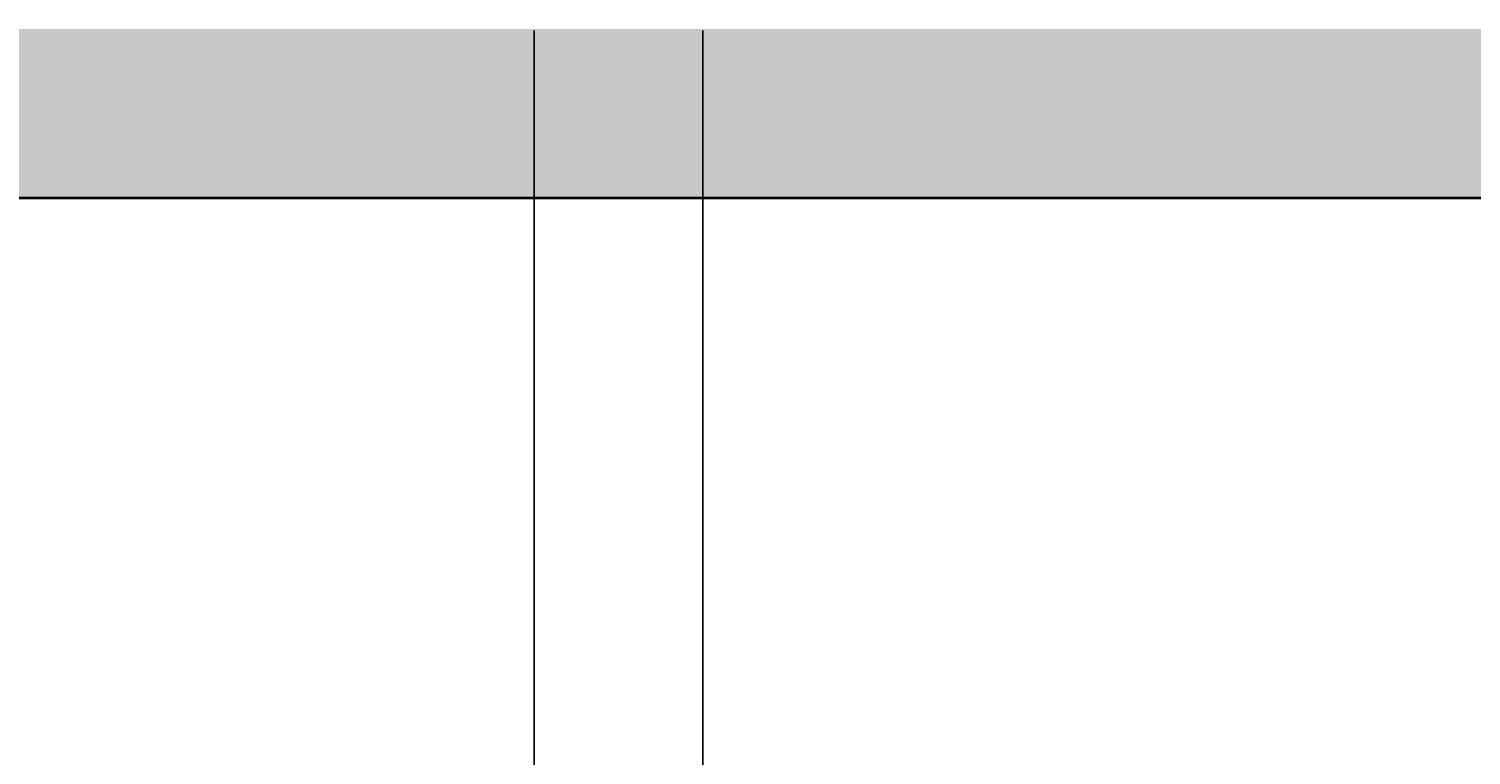
# Model space of a CAD drawing. Units: inches. Extents: x 2549 to 3108, y 1683 to 2362.
# Tile 15 of 30: x 2711 to 2762, y 2055 to 2081. Entities that reach past the tile are written whole.
import ezdxf

# ---------------------------------------------------------------- set-up
doc = ezdxf.new("R2010")
doc.units = ezdxf.units.IN
for name, color, linetype, lineweight in [('A-ANNO-DIMS', 2, 'Continuous', 18), ('A-WALL', 7, 'Continuous', 35), ('A-WALL-PATT', 89, 'Continuous', 13)]:
    doc.layers.add(name, color=color, linetype=linetype, lineweight=lineweight)
doc.layers.add('C-PKNG-VEHI-PATT', color=251, linetype='Continuous', lineweight=13, true_color=0x636466)
doc.layers.add('C-PVMT-PATT', color=9, linetype='Continuous', lineweight=13, true_color=0xc7c8ca)
doc.styles.get("Standard").update_dxf_attribs({"font": 'arial.ttf'})
doc.dimstyles.get("Standard").update_dxf_attribs({"dimtxt": 0.18, "dimasz": 0.18, "dimexe": 0.18, "dimexo": 0.0625, "dimgap": 0.09, "dimtad": 0, "dimtih": 1, "dimtoh": 1, "dimdec": 4, "dimzin": 0, "dimdsep": 46, "dimtxsty": 'Standard', "dimcen": 0.09, "dimadec": 0, "dimazin": 0, "dimtfac": 1, "dimtdec": 4, "dimtofl": 0, "dimtmove": 0, "dimatfit": 3, "dimfxl": 1, "dimtolj": 1, "dimtzin": 0, "dimarcsym": 0})

# ---------------------------------------------------------------- blocks, each defined once
blk = doc.blocks.new('*D42')
at = {"layer": 'A-ANNO-DIMS', "color": 0, "lineweight": -2, "transparency": 16777216}
for p, q in [((2638.643, 2080.461), (2638.643, 1683.444)), ((2728.643, 2080.461), (2728.643, 1683.444)), ((2638.823, 1683.624), (2683.424, 1683.624)), ((2728.463, 1683.624), (2683.861, 1683.624))]:
    blk.add_line(p, q, dxfattribs=at)
at = {"layer": 'A-ANNO-DIMS', "color": 0, "transparency": 16777216}
for points in [[(2638.823, 1683.654), (2638.823, 1683.594), (2638.643, 1683.624)], [(2728.463, 1683.654), (2728.463, 1683.594), (2728.643, 1683.624)]]:
    blk.add_solid(points, dxfattribs=at)
at = {"layer": 'Defpoints', "color": 0, "transparency": 16777216}
for p in [(2638.643, 2080.524), (2728.643, 2080.524), (2728.643, 1683.624)]:
    blk.add_point(p, dxfattribs=at)
at = {"layer": 'A-ANNO-DIMS', "color": 0, "transparency": 16777216, "insert": (2683.643, 1683.624), "char_height": 0.18, "attachment_point": 5}
blk.add_mtext('\\A1;90', dxfattribs=at)
blk = doc.blocks.new('*D43')
at = {"layer": 'A-ANNO-DIMS', "color": 0, "lineweight": -2, "transparency": 16777216}
for p, q in [((2734.643, 2080.461), (2734.643, 1683.444)), ((2806.643, 2080.461), (2806.643, 1683.444)), ((2734.823, 1683.624), (2770.425, 1683.624)), ((2806.463, 1683.624), (2770.86, 1683.624))]:
    blk.add_line(p, q, dxfattribs=at)
at = {"layer": 'A-ANNO-DIMS', "color": 0, "transparency": 16777216}
for points in [[(2734.823, 1683.654), (2734.823, 1683.594), (2734.643, 1683.624)], [(2806.463, 1683.654), (2806.463, 1683.594), (2806.643, 1683.624)]]:
    blk.add_solid(points, dxfattribs=at)
at = {"layer": 'Defpoints', "color": 0, "transparency": 16777216}
for p in [(2734.643, 2080.524), (2806.643, 2080.524), (2806.643, 1683.624)]:
    blk.add_point(p, dxfattribs=at)
at = {"layer": 'A-ANNO-DIMS', "color": 0, "transparency": 16777216, "insert": (2770.643, 1683.624), "char_height": 0.18, "attachment_point": 5}
blk.add_mtext('\\A1;72', dxfattribs=at)
blk = doc.blocks.new('*D59')
at = {"layer": 'A-ANNO-DIMS', "color": 0, "lineweight": -2, "transparency": 16777216}
for p, q in [((2680.978, 1761.586), (2680.978, 2362.323)), ((2786.158, 1761.586), (2786.158, 2362.323)), ((2681.158, 2362.143), (2733.112, 2362.143)), ((2785.978, 2362.143), (2734.023, 2362.143))]:
    blk.add_line(p, q, dxfattribs=at)
at = {"layer": 'A-ANNO-DIMS', "color": 0, "transparency": 16777216}
for points in [[(2681.158, 2362.173), (2681.158, 2362.113), (2680.978, 2362.143)], [(2785.978, 2362.173), (2785.978, 2362.113), (2786.158, 2362.143)]]:
    blk.add_solid(points, dxfattribs=at)
at = {"layer": 'Defpoints', "color": 0, "transparency": 16777216}
for p in [(2786.158, 2362.143), (2680.978, 1761.524), (2786.158, 1761.524)]:
    blk.add_point(p, dxfattribs=at)
at = {"layer": 'A-ANNO-DIMS', "color": 0, "transparency": 16777216, "insert": (2733.568, 2362.143), "char_height": 0.18, "attachment_point": 5}
blk.add_mtext('\\A1;105.18', dxfattribs=at)

msp = doc.modelspace()

# ---------------------------------------------------------------- hatches: boundary and pattern name
at = {"layer": 'A-WALL-PATT'}
h = msp.add_hatch(color=256, dxfattribs=at)
h.dxf.hatch_style = 1
h.paths.add_polyline_path([(2638.6427, 2272.5237), (3034.6427, 2272.5237), (3034.6427, 1936.5237), (3043.6427, 1936.5237), (3043.6427, 2281.5237), (2629.6427, 2281.5237), (2629.6427, 2074.5237), (2812.6427, 2074.5237), (2812.6427, 2140.5237), (2785.7177, 2140.5237), (2785.7177, 2134.5237), (2806.6427, 2134.5237), (2806.6427, 2080.5237), (2638.6427, 2080.5237)])
h.paths.add_polyline_path([(2638.6427, 1972.5237), (2662.6427, 1972.5237), (2662.6427, 2041.0557), (2653.6427, 2041.0557), (2653.6427, 1978.5237), (2629.6427, 1978.5237), (2629.6427, 1795.5237), (2662.6427, 1795.5237), (2881.6427, 1795.5237), (2881.6427, 1936.5237), (2965.9351, 1936.5237), (2965.9351, 1974.5439), (2959.9351, 1974.5439), (2959.9351, 1945.5237), (2881.6427, 1945.5237), (2872.6427, 1945.5237), (2872.6427, 1804.5237), (2662.6427, 1804.5237), (2638.6427, 1804.5237)])
at = {"layer": 'C-PKNG-VEHI-PATT'}
h = msp.add_hatch(color=256, dxfattribs=at)
h.dxf.hatch_style = 1
edge = h.paths.add_edge_path()
edge.add_ellipse((2935.7258, 1791.964), major_axis=(-50.66, 0), ratio=0.8423039, start_angle=248.16505, end_angle=265.72258)
edge.add_line((2938.911, 1834.5507), (2925.8653, 1834.5507))
edge.add_ellipse((2929.0505, 1791.964), major_axis=(50.66, 0), ratio=0.8423039, start_angle=94.27742, end_angle=111.83495)
edge.add_line((2912.8508, 1832.3947), (2914.2044, 1822.2495))
edge.add_ellipse((2930.6538, 1783.1023), major_axis=(-49.3014, 0), ratio=0.8423039, start_angle=-85.12993, end_angle=-67.20809, ccw=False)
edge.add_line((2927.1247, 1824.5225), (2937.6516, 1824.5225))
edge.add_ellipse((2934.1225, 1783.1023), major_axis=(49.3014, 0), ratio=0.8423039, start_angle=67.20809, end_angle=85.12993, ccw=False)
edge.add_line((2950.5719, 1822.2495), (2951.9255, 1832.3947))
edge = h.paths.add_edge_path()
edge.add_ellipse((2903.4793, 1857.3351), major_axis=(-34.7979, 0), ratio=0.8423039, start_angle=180, end_angle=209.43857)
edge.add_ellipse((2961.297, 1857.3351), major_axis=(34.7979, 0), ratio=0.8423039, start_angle=150.56143, end_angle=180)
edge.add_line((2926.4991, 1857.3351), (2926.4991, 1843.7609))
edge.add_ellipse((2924.1251, 1844.3143), major_axis=(-0.2209, 3.9278), ratio=0.6038336, start_angle=89.00201, end_angle=253.65741, ccw=False)
edge.add_line((2921.7512, 1844.2222), (2921.7512, 1853.3975))
edge.add_line((2921.7512, 1853.3975), (2925.269, 1855.8484))
edge.add_ellipse((2925.4782, 1855.4931), major_axis=(0.4584, 0), ratio=0.8423039, start_angle=90, end_angle=134.48021, ccw=False)
edge.add_line((2925.4782, 1855.8792), (2926.4991, 1855.8792))
edge.add_line((2926.4991, 1855.8792), (2926.4991, 1857.3351))
edge.add_ellipse((2961.297, 1857.3351), major_axis=(34.7979, 0), ratio=0.8423039, start_angle=150.56143, end_angle=180, ccw=False)
edge.add_line((2932.3882, 1873.6501), (2932.3882, 1875.7801))
edge.add_ellipse((2932.3882, 1875.3939), major_axis=(0.4584, 0), ratio=0.8423039, start_angle=90, end_angle=127.93313)
edge.add_line((2932.1366, 1875.7167), (2928.5915, 1873.7564))
edge.add_ellipse((2899.9271, 2002.4692), major_axis=(155.4756, 0), ratio=0.84230387, start_angle=-80.743434, end_angle=-77.445067, ccw=False)
edge.add_ellipse((2949.4402, 1715.2151), major_axis=(-189.1422, 0), ratio=0.84230387, start_angle=-79.790461, end_angle=-77.555373)
edge.add_ellipse((3300.3614, 1852.5642), major_axis=(-386.1662, 0), ratio=0.84230387, start_angle=-2.863715, end_angle=2.198541)
edge.add_ellipse((2929.0505, 1792.5159), major_axis=(-55.6192, 0), ratio=0.8423039, start_angle=-85.91759, end_angle=-72.28005, ccw=False)
edge.add_line((2925.7129, 1839.2798), (2939.0634, 1839.2798))
edge.add_ellipse((2935.7258, 1792.5159), major_axis=(55.6192, 0), ratio=0.8423039, start_angle=72.28005, end_angle=85.91759, ccw=False)
edge.add_ellipse((2564.4149, 1852.5642), major_axis=(-386.1662, 0), ratio=0.84230387, start_angle=177.801459, end_angle=182.863715)
edge.add_ellipse((2915.3361, 1715.2151), major_axis=(189.1422, 0), ratio=0.84230387, start_angle=77.555373, end_angle=79.790461)
edge.add_ellipse((2964.8492, 2002.4692), major_axis=(-155.4756, 0), ratio=0.84230387, start_angle=77.445067, end_angle=80.743434, ccw=False)
edge.add_line((2936.1848, 1873.7564), (2932.6397, 1875.7167))
edge.add_ellipse((2932.3882, 1875.3939), major_axis=(0.4584, 0), ratio=0.8423039, start_angle=52.06687, end_angle=90)
edge.add_line((2932.3882, 1875.7801), (2932.3882, 1873.6501))
edge.add_ellipse((2903.4793, 1857.3351), major_axis=(-34.7979, 0), ratio=0.8423039, start_angle=180, end_angle=209.43857, ccw=False)
edge.add_line((2938.2772, 1857.3351), (2938.2772, 1855.8792))
edge.add_line((2938.2772, 1855.8792), (2939.4059, 1855.8792))
edge.add_ellipse((2939.2981, 1855.4931), major_axis=(-0.4584, 0), ratio=0.8423039, start_angle=225.51979, end_angle=270, ccw=False)
edge.add_line((2939.5903, 1855.7906), (2943.0251, 1853.3975))
edge.add_line((2943.0251, 1853.3975), (2943.0251, 1844.2222))
edge.add_ellipse((2940.6512, 1844.3143), major_axis=(0.2209, 3.9278), ratio=0.6038336, start_angle=106.34259, end_angle=270.99799, ccw=False)
edge.add_line((2938.2772, 1843.7609), (2938.2772, 1857.3351))
edge = h.paths.add_edge_path()
edge.add_ellipse((2932.3882, 1865.1973), major_axis=(91.081, 0), ratio=0.8423039, start_angle=256.401865, end_angle=283.598135, ccw=False)
edge.add_line((2914.2044, 1790.0239), (2914.2044, 1778.3622))
edge.add_ellipse((2932.3882, 1853.5356), major_axis=(91.081, 0), ratio=0.8423039, start_angle=256.401865, end_angle=283.598135)
edge.add_line((2950.5719, 1778.3622), (2950.5719, 1790.0239))
edge = h.paths.add_edge_path()
edge.add_ellipse((2948.7383, 1772.3145), major_axis=(1.8336, 0), ratio=0.8423039, start_angle=0, end_angle=90)
edge.add_line((2948.7383, 1773.859), (2916.038, 1773.859))
edge.add_ellipse((2916.038, 1772.3145), major_axis=(1.8336, 0), ratio=0.8423039, start_angle=90, end_angle=180)
edge.add_line((2914.2044, 1772.3145), (2914.2044, 1760.2558))
edge.add_line((2914.2044, 1760.2558), (2950.5719, 1760.2558))
edge.add_line((2950.5719, 1760.2558), (2950.5719, 1772.3145))
h.paths.add_polyline_path([(2748.8496, 2101.6383), (2798.148, 2101.6383), (2798.148, 2111.4248), (2748.8496, 2111.4248)], flags=9)
h.paths.add_polyline_path([(2685.2081, 2101.489), (2719.3253, 2101.489), (2719.3253, 2111.2819), (2685.2081, 2111.2819)], flags=9)
h.paths.add_polyline_path([(2814.6852, 1907.1328), (2847.8384, 1907.1328), (2847.8384, 1916.9258), (2814.6852, 1916.9258)], flags=9)
h.paths.add_polyline_path([(2814.3906, 1835.5864), (2848.0172, 1835.5864), (2848.0172, 1845.3794), (2814.3906, 1845.3794)], flags=9)
h.paths.add_polyline_path([(2800.5245, 1759.1674), (2853.7435, 1759.1674), (2853.7435, 1768.954), (2800.5245, 1768.954)], flags=9)
h.paths.add_polyline_path([(2972.4611, 1807.3305), (3015.3943, 1807.3305), (3015.3943, 1817.117), (2972.4611, 1817.117)], flags=9)
h.paths.add_polyline_path([(2902.3327, 1888.6731), (2937.9131, 1888.6731), (2937.9131, 1898.4661), (2902.3327, 1898.4661)], flags=9)
h.paths.add_polyline_path([(2712.1779, 1878.9039), (2754.1257, 1878.9039), (2754.1257, 1888.6904), (2712.1779, 1888.6904)], flags=9)
h.paths.add_polyline_path([(2614.0056, 2012.812), (2650.0251, 2012.812), (2650.0251, 2022.4371), (2614.0056, 2022.4371)], flags=9)
h.paths.add_polyline_path([(2713.3129, 2003.1645), (2747.4237, 2003.1645), (2747.4237, 2012.951), (2713.3129, 2012.951)], flags=9)
h.paths.add_polyline_path([(2950.1379, 2001.6934), (2982.2992, 2001.6934), (2982.2992, 2011.48), (2950.1379, 2011.48)], flags=9)
h.paths.add_polyline_path([(2940.864, 2238.5537), (2997.5066, 2238.5537), (2997.5066, 2248.3466), (2940.864, 2248.3466)], flags=9)
h.paths.add_polyline_path([(2821.5457, 2202.8348), (2855.663, 2202.8348), (2855.663, 2212.6278), (2821.5457, 2212.6278)], flags=9)
h.paths.add_polyline_path([(2661.8026, 2238.6249), (2718.4451, 2238.6249), (2718.4451, 2248.4179), (2661.8026, 2248.4179)], flags=9)
at = {"layer": 'C-PVMT-PATT'}
h = msp.add_hatch(color=256, dxfattribs=at)
h.dxf.hatch_style = 1
h.paths.add_polyline_path([(3067.6427, 2305.5237), (2605.6427, 2305.5237), (2605.6427, 2074.5237), (2629.6427, 2074.5237), (2629.6427, 2281.5237), (3043.6427, 2281.5237), (3043.6427, 1885.5237), (3043.6427, 1872.8745), (3031.1672, 1872.8745), (3031.1672, 1862.5731), (2995.8054, 1862.5731), (2995.8054, 1872.8745), (2983.1752, 1872.8745), (2983.1752, 1885.5237), (2881.6427, 1885.5237), (2881.6427, 1795.5237), (2751.0977, 1795.5237), (2751.0977, 1761.5237), (2786.1577, 1761.5237), (2786.1577, 1723.5237), (2881.84, 1723.5237), (2881.84, 1714.5237), (3067.6427, 1714.5237), (3067.6427, 1723.5237)])
edge = h.paths.add_edge_path(flags=16)
edge.add_ellipse((2949.4402, 1710.9683), major_axis=(-194.1014, 0), ratio=0.84230387, start_angle=-77.874034, end_angle=-76.219471, ccw=False)
edge.add_ellipse((2949.4402, 1715.2151), major_axis=(-189.1422, 0), ratio=0.84230387, start_angle=-79.790461, end_angle=-77.555373, ccw=False)
edge.add_ellipse((2899.9271, 2002.4692), major_axis=(155.4756, 0), ratio=0.84230387, start_angle=-80.743434, end_angle=-77.445067)
edge.add_line((2928.5915, 1873.7564), (2932.3882, 1875.8558))
edge.add_line((2932.3882, 1875.8558), (2936.1848, 1873.7564))
edge.add_ellipse((2964.8492, 2002.4692), major_axis=(-155.4756, 0), ratio=0.84230387, start_angle=77.445067, end_angle=80.743434)
edge.add_ellipse((2915.3361, 1715.2151), major_axis=(189.1422, 0), ratio=0.84230387, start_angle=77.555373, end_angle=79.790461, ccw=False)
edge.add_ellipse((2915.3361, 1710.9683), major_axis=(-194.1014, 0), ratio=0.84230387, start_angle=256.219471, end_angle=257.874034, ccw=False)
edge.add_ellipse((2628.2871, 1850.2612), major_axis=(-327.2532, 0), ratio=0.84230387, start_angle=182.17995, end_angle=183.650428, ccw=False)
edge.add_ellipse((2955.5637, 1861.9334), major_axis=(-0.9168, 0), ratio=0.8423039, start_angle=180, end_angle=270, ccw=False)
edge.add_line((2956.4805, 1862.3857), (2956.4805, 1846.4866))
edge.add_ellipse((2955.5637, 1846.939), major_axis=(-0.9168, 0), ratio=0.8423039, start_angle=90, end_angle=180, ccw=False)
edge.add_ellipse((-3607.0606, 1835.832), major_axis=(-6562.6242, 0), ratio=0.84230387, start_angle=179.61613322, end_angle=180.09022909, ccw=False)
edge.add_ellipse((2955.5637, 1791.0926), major_axis=(0.9168, 0), ratio=0.8423039, start_angle=0, end_angle=90, ccw=False)
edge.add_line((2956.4805, 1791.545), (2956.4805, 1775.6459))
edge.add_ellipse((2955.5637, 1776.0982), major_axis=(0.9168, 0), ratio=0.8423039, start_angle=270, end_angle=360, ccw=False)
edge.add_ellipse((-3607.0606, 1835.832), major_axis=(-6562.6242, 0), ratio=0.84230387, start_angle=179.3813568, end_angle=179.47172853, ccw=False)
edge.add_ellipse((2954.5907, 1763.8768), major_axis=(-1.3752, 0), ratio=0.8423039, start_angle=179.37176, end_angle=248.46476, ccw=False)
edge.add_ellipse((-3607.519, 1835.832), major_axis=(-6564.0409, 0), ratio=0.842303863, start_angle=179.35344594, end_angle=179.37176282, ccw=False)
edge.add_ellipse((2952.6829, 1761.8002), major_axis=(3.2503, 0), ratio=0.8423039, start_angle=-90, end_angle=-0.64655, ccw=False)
edge.add_line((2952.6829, 1759.0625), (2912.0934, 1759.0625))
edge.add_ellipse((2912.0934, 1761.8002), major_axis=(3.2503, 0), ratio=0.8423039, start_angle=180.64655, end_angle=270, ccw=False)
edge.add_ellipse((9472.2953, 1835.832), major_axis=(-6564.0409, 0), ratio=0.842303871, start_angle=0.62823722, end_angle=0.6465541, ccw=False)
edge.add_ellipse((2910.1856, 1763.8768), major_axis=(1.3752, 0), ratio=0.8423039, start_angle=111.53524, end_angle=180.62824, ccw=False)
edge.add_ellipse((9471.8369, 1835.832), major_axis=(-6562.6242, 0), ratio=0.84230387, start_angle=0.52827147, end_angle=0.6465541, ccw=False)
edge.add_ellipse((2909.2126, 1776.0982), major_axis=(-0.9168, 0), ratio=0.8423039, start_angle=0, end_angle=90, ccw=False)
edge.add_line((2908.2958, 1775.6459), (2908.2958, 1791.545))
edge.add_ellipse((2909.2126, 1791.0926), major_axis=(-0.9168, 0), ratio=0.8423039, start_angle=-90, end_angle=0, ccw=False)
edge.add_ellipse((9471.8369, 1835.832), major_axis=(-6562.6242, 0), ratio=0.84230387, start_angle=-0.09022909, end_angle=0.38386678, ccw=False)
edge.add_ellipse((2909.2126, 1846.939), major_axis=(-0.9168, 0), ratio=0.8423039, start_angle=0, end_angle=90, ccw=False)
edge.add_line((2908.2958, 1846.4866), (2908.2958, 1862.3857))
edge.add_ellipse((2909.2126, 1861.9334), major_axis=(0.9168, 0), ratio=0.8423039, start_angle=90, end_angle=180, ccw=False)
edge.add_ellipse((3236.4892, 1850.2612), major_axis=(327.2532, 0), ratio=0.84230387, start_angle=176.349572, end_angle=177.82005, ccw=False)
edge = h.paths.add_edge_path(flags=0)
edge.add_ellipse((2903.4793, 1857.3351), major_axis=(-34.7979, 0), ratio=0.8423039, start_angle=180, end_angle=209.43857, ccw=False)
edge.add_line((2938.2772, 1857.3351), (2938.2772, 1855.8792))
edge.add_line((2938.2772, 1855.8792), (2939.4631, 1855.8792))
edge.add_line((2939.4631, 1855.8792), (2943.0251, 1853.3975))
edge.add_line((2943.0251, 1853.3975), (2943.0251, 1844.2222))
edge.add_ellipse((2940.6512, 1844.3143), major_axis=(0.2209, 3.9278), ratio=0.6038336, start_angle=106.34259, end_angle=270.99799, ccw=False)
edge.add_line((2938.2772, 1843.7609), (2938.2772, 1857.3351))
edge.add_ellipse((2903.4793, 1857.3351), major_axis=(-34.7979, 0), ratio=0.8423039, start_angle=180, end_angle=209.43857)
edge.add_ellipse((2961.297, 1857.3351), major_axis=(34.7979, 0), ratio=0.8423039, start_angle=150.56143, end_angle=180)
edge.add_line((2926.4991, 1857.3351), (2926.4991, 1843.7609))
edge.add_ellipse((2924.1251, 1844.3143), major_axis=(-0.2209, 3.9278), ratio=0.6038336, start_angle=89.00201, end_angle=253.65741, ccw=False)
edge.add_line((2921.7512, 1844.2222), (2921.7512, 1853.3975))
edge.add_line((2921.7512, 1853.3975), (2925.3132, 1855.8792))
edge.add_line((2925.3132, 1855.8792), (2926.4991, 1855.8792))
edge.add_line((2926.4991, 1855.8792), (2926.4991, 1857.3351))
edge.add_ellipse((2961.297, 1857.3351), major_axis=(34.7979, 0), ratio=0.8423039, start_angle=150.56143, end_angle=180, ccw=False)
edge = h.paths.add_edge_path(flags=0)
edge.add_ellipse((2929.0505, 1791.964), major_axis=(50.66, 0), ratio=0.8423039, start_angle=94.27742, end_angle=111.83495, ccw=False)
edge.add_line((2925.8653, 1834.5507), (2938.911, 1834.5507))
edge.add_ellipse((2935.7258, 1791.964), major_axis=(-50.66, 0), ratio=0.8423039, start_angle=248.16505, end_angle=265.72258, ccw=False)
edge.add_line((2951.9255, 1832.3947), (2950.5719, 1822.2495))
edge.add_ellipse((2934.1225, 1783.1023), major_axis=(49.3014, 0), ratio=0.8423039, start_angle=67.20809, end_angle=85.12993)
edge.add_line((2937.6516, 1824.5225), (2927.1247, 1824.5225))
edge.add_ellipse((2930.6538, 1783.1023), major_axis=(-49.3014, 0), ratio=0.8423039, start_angle=-85.12993, end_angle=-67.20809)
edge.add_line((2914.2044, 1822.2495), (2912.8508, 1832.3947))
edge = h.paths.add_edge_path(flags=0)
edge.add_line((2910.1338, 1829.4651), (2912.6432, 1821.2711))
edge.add_ellipse((5203.7787, 1816.4367), major_axis=(-2291.1426, 0), ratio=0.84230387, start_angle=-0.1208974, end_angle=0.3640763)
edge.add_line((2912.7012, 1801.8782), (2910.3305, 1792.5698))
edge.add_ellipse((9471.8369, 1835.832), major_axis=(-6561.7074, 0), ratio=0.84230387, start_angle=0.05559431, end_angle=0.37776419, ccw=False)
edge = h.paths.add_edge_path(flags=0)
edge.add_ellipse((-3607.0606, 1835.832), major_axis=(6561.7074, 0), ratio=0.84230387, start_angle=-0.37776419, end_angle=-0.05559431, ccw=False)
edge.add_line((2954.4458, 1792.5698), (2952.0751, 1801.8782))
edge.add_ellipse((660.9976, 1816.4367), major_axis=(2291.1426, 0), ratio=0.84230387, start_angle=-0.3640763, end_angle=0.1208974)
edge.add_line((2952.1331, 1821.2711), (2954.6425, 1829.4651))
edge = h.paths.add_edge_path(flags=0)
edge.add_ellipse((2932.3882, 1865.1973), major_axis=(91.081, 0), ratio=0.8423039, start_angle=256.401865, end_angle=283.598135)
edge.add_line((2950.5719, 1790.0239), (2950.5719, 1778.3622))
edge.add_ellipse((2932.3882, 1853.5356), major_axis=(91.081, 0), ratio=0.8423039, start_angle=256.401865, end_angle=283.598135, ccw=False)
edge.add_line((2914.2044, 1778.3622), (2914.2044, 1790.0239))
edge = h.paths.add_edge_path(flags=0)
edge.add_line((2916.038, 1773.859), (2948.7383, 1773.859))
edge.add_ellipse((2948.7383, 1772.3145), major_axis=(1.8336, 0), ratio=0.8423039, start_angle=0, end_angle=90, ccw=False)
edge.add_line((2950.5719, 1772.3145), (2950.5719, 1760.2558))
edge.add_line((2950.5719, 1760.2558), (2914.2044, 1760.2558))
edge.add_line((2914.2044, 1760.2558), (2914.2044, 1772.3145))
edge.add_ellipse((2916.038, 1772.3145), major_axis=(1.8336, 0), ratio=0.8423039, start_angle=90, end_angle=180, ccw=False)
h.paths.add_polyline_path([(2629.6427, 1978.5237), (2605.6427, 1978.5237), (2605.6427, 1723.5237), (2629.6427, 1723.5237), (2629.6427, 1795.5237)], flags=17)
h.paths.add_polyline_path([(2800.5245, 1759.1674), (2853.7435, 1759.1674), (2853.7435, 1768.954), (2800.5245, 1768.954)], flags=24)
h.paths.add_polyline_path([(2972.4611, 1807.3305), (3015.3943, 1807.3305), (3015.3943, 1817.117), (2972.4611, 1817.117)], flags=24)

# ---------------------------------------------------------------- linework, layer by layer
at = {"layer": 'A-WALL'}
msp.add_line((2629.6427, 2074.5237), (2812.6427, 2074.5237), dxfattribs=at)

# ---------------------------------------------------------------- dimensions: what is measured, and where the dimension line sits
at = {"layer": 'A-ANNO-DIMS'}
for base, p1, p2, override, picture, middle in [((2786.1577, 2362.1425), (2680.9778, 1761.5237), (2786.1577, 1761.5237), {"dimdec": 2, "dimlfac": 1, "dimrnd": 0, "dimzin": 0, "dimdsep": 46, "dimlunit": 2}, '*D59', (2733.5678, 2362.1425)), ((2728.6427, 1683.6237), (2638.6427, 2080.5237), (2728.6427, 2080.5237), {"dimdec": 0, "dimlfac": 1, "dimrnd": 0, "dimzin": 0, "dimdsep": 46, "dimlunit": 2}, '*D42', (2683.6427, 1683.6237)), ((2806.6427, 1683.6237), (2734.6427, 2080.5237), (2806.6427, 2080.5237), {"dimdec": 0, "dimlfac": 1, "dimrnd": 0, "dimzin": 0, "dimdsep": 46, "dimlunit": 2}, '*D43', (2770.6427, 1683.6237))]:
    dim = msp.add_linear_dim(base=base, p1=p1, p2=p2, dimstyle='Standard', override=override, dxfattribs=at)
    dim.commit()
    dim.dimension.update_dxf_attribs({"geometry": picture, "text_midpoint": middle})

doc.saveas('drawing.dxf')
